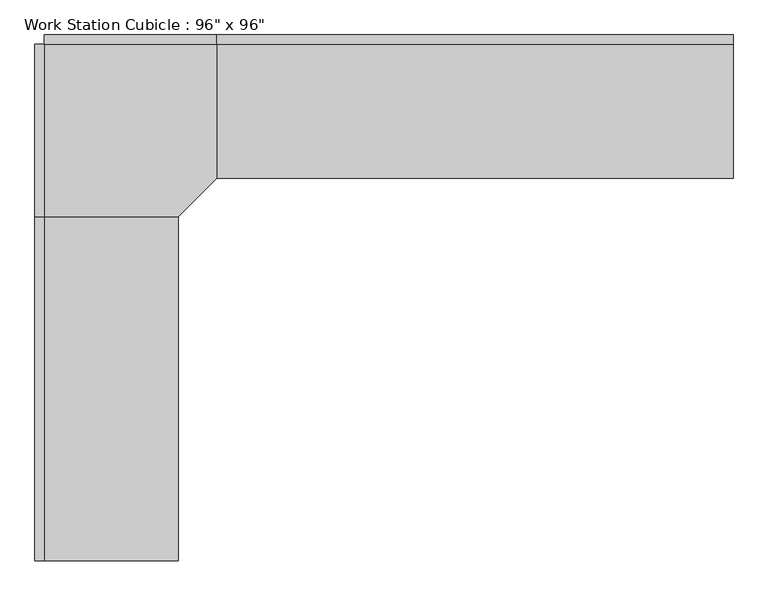
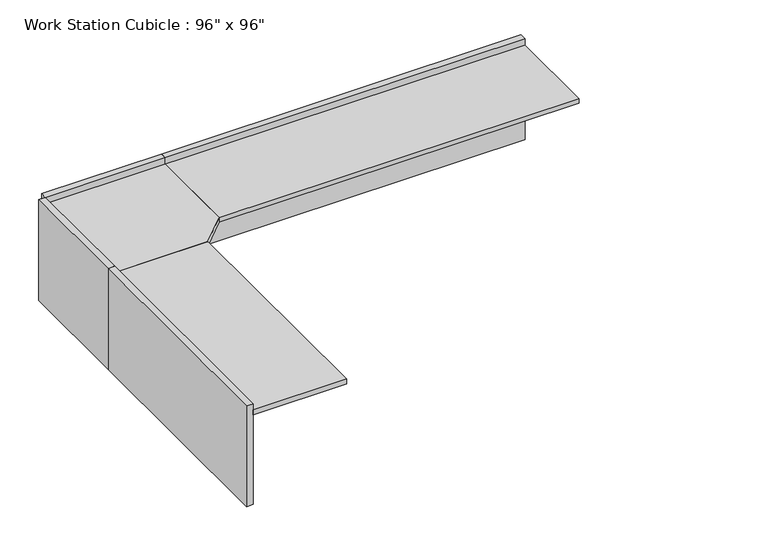
"""IFC4 building model written with IfcOpenShell, lengths in millimetres: furniture geometry."""

from ifc_helpers import new_model, si_unit, frame, origin, origin_with_axes, place, context, project, spatial, polyline, outline, extrude, source, transform, mapped, element, save


def furniture_452c495f(model_context):
    return source(origin(), model_context, "Body", "SweptSolid", [
        extrude(outline(polyline([(-80.9317522, -545.8230076), (833.4682478, -545.8230076), (833.4682478, -1257.0230076), (630.2682478, -1460.2230076), (-80.9317522, -1460.2230076), (-80.9317522, -545.8230076)])), frame((0.0, 0.0, 723.9), z_axis=(0.0, 0.0, 1.0), x_axis=(1.0, 0.0, 0.0)), (0.0, 0.0, 1.0), 38.1),
        extrude(outline(polyline([(630.2682478, -3289.0230076), (-80.9317522, -3289.0230076), (-80.9317522, -1460.2230076), (630.2682478, -1460.2230076), (630.2682478, -3289.0230076)])), frame((0.0, 0.0, 723.9), z_axis=(0.0, 0.0, 1.0), x_axis=(1.0, 0.0, 0.0)), (0.0, 0.0, 1.0), 38.1),
        extrude(outline(polyline([(3576.6682478, -1257.0230076), (833.4682478, -1257.0230076), (833.4682478, -545.8230076), (3576.6682478, -545.8230076), (3576.6682478, -1257.0230076)])), frame((0.0, 0.0, 723.9), z_axis=(0.0, 0.0, 1.0), x_axis=(1.0, 0.0, 0.0)), (0.0, 0.0, 1.0), 38.1),
        extrude(outline(polyline([(3576.6682478, -545.8230076), (833.4682478, -545.8230076), (833.4682478, -495.0230076), (3576.6682478, -495.0230076), (3576.6682478, -545.8230076)])), origin_with_axes(), (0.0, 0.0, 1.0), 812.8),
        extrude(outline(polyline([(833.4682478, -545.8230076), (-80.9317522, -545.8230076), (-80.9317522, -495.0230076), (833.4682478, -495.0230076), (833.4682478, -545.8230076)])), origin_with_axes(), (0.0, 0.0, 1.0), 812.8),
        extrude(outline(polyline([(-80.9317522, -1460.2230076), (-131.7317522, -1460.2230076), (-131.7317522, -545.8230076), (-80.9317522, -545.8230076), (-80.9317522, -1460.2230076)])), origin_with_axes(), (0.0, 0.0, 1.0), 812.8),
        extrude(outline(polyline([(-80.9317522, -3289.0230076), (-131.7317522, -3289.0230076), (-131.7317522, -1460.2230076), (-80.9317522, -1460.2230076), (-80.9317522, -3289.0230076)])), origin_with_axes(), (0.0, 0.0, 1.0), 812.8),
    ])


if __name__ == "__main__":
    model = new_model("IFC4")
    model_context = context("Model", 3, world=origin())
    ifc_project = project(units=[si_unit("LENGTHUNIT", "METRE", prefix="MILLI")], contexts=[model_context])
    site = spatial("IfcSite", under=ifc_project)
    building = spatial("IfcBuilding", under=site)
    placement = place(None, origin())
    furniture_shape = furniture_452c495f(model_context)
    element("IfcFurniture", 1, ObjectType="Work Station Cubicle : 96\" x 96\"", at=placement, inside=building, context=model_context, shape_type="MappedRepresentation", body=[
        mapped(furniture_shape, transform((0.0, 0.0, 0.0), x_axis=(1.0, 0.0, 0.0), y_axis=(0.0, 1.0, 0.0), z_axis=(0.0, 0.0, 1.0))),
    ])
    save(model, "model.ifc")

# Revit data of these elements
# Type "Work Station Cubicle : 96\" x 96\""
#   Assembly Code = "E2020"
#   Desktop Height = 2' - 6"
#   Desktop1 Width = 2' - 4"
#   Desktop2 Width = 2' - 4"
#   Panel Height = 2' - 8"
#   Panel1 Length = 6' - 0"
#   Panel2 Length = 9' - 0"
#   Cube Panel Material = Textile - Light Gray
#   Work Top Material = Laminate, Ivory, Matte
#   Default Elevation = 0
# Element 1 (IfcFurniture, "Work Station Cubicle : 96\" x 96\"")
#   Materials on its faces: "Textile - Light Gray", "Laminate, Ivory, Matte"
# Materials
#   "Textile - Light Gray": class "Fabric", colour RGB 204 204 204, transparency 0
#   "Laminate, Ivory, Matte": class "Plastic", colour RGB 247 247 239, transparency 0, Description = "Plastic Laminate - Ivory, Matte", Cost = 0
